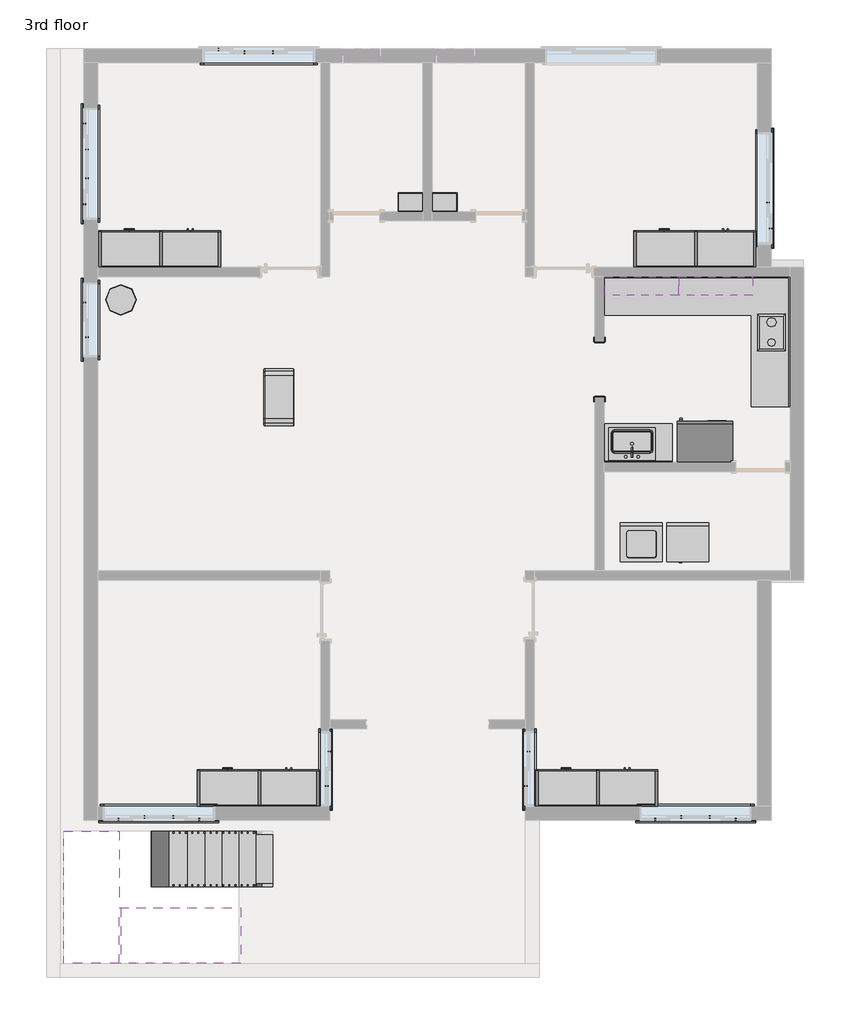
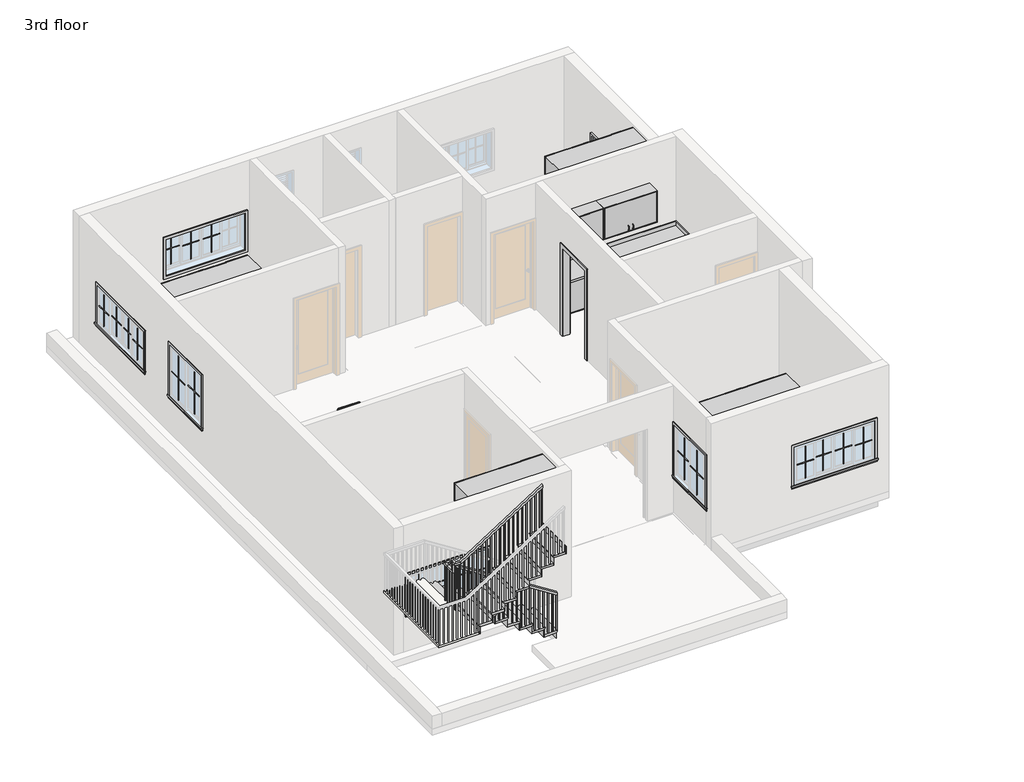
# One storey, part 3 of 4: 42 proxies, 15 furniture elements, 3 flow terminals, 2 stair flights, 1 railing, 1 slab.
"""IFC4 building model written with IfcOpenShell, lengths in millimetres."""

from ifc_helpers import new_model, si_unit, frame, origin, place, context, project, spatial, polyline, outline, extrude, faceted_brep, transform, mapped, element, save
from components import proxy_3c1fa1d0, proxy_97c73763, muntin_pattern_2x2_muntin_pattern_2x2_c2d27229, muntin_pattern_2x2_muntin_pattern_2x2_cf37b409, muntin_pattern_2x2_muntin_pattern_2x2_31a16349, proxy_7dd6dadb, trim_window_exterior_flat_with_sill_ac84ebb5, trim_window_exterior_flat_with_sill_7cfdd449, trim_window_exterior_flat_with_sill_3c945769, trim_window_interior_flat_picture_frame_caf2db4f, trim_window_interior_flat_picture_frame_f1e0b15b, trim_window_interior_flat_picture_frame_0edfbaa2, proxy_e75280ca, flow_terminal_7145266d, flow_terminal_4d548711, furniture_2dca108f, furniture_65fa61b5, furniture_1wardrobe_6271_1wardrobe_6271_4dd35231, furniture_3428e43d, furniture_bf8a676d, furniture_97fe820d, furniture_a6d59748, furniture_f5a42f9b, furniture_9d41381f, furniture_ea954fa4, non_monolithic_landing_543f77e1, stair_flight_6f06193a, stair_flight_13cb1edf

model = new_model("IFC4")

# Units and contexts
model_context = context("Model", 3, world=origin())
ifc_project = project(units=[si_unit("LENGTHUNIT", "METRE", prefix="MILLI")], contexts=[model_context])

# Site, building, storey
site = spatial("IfcSite", under=ifc_project)
building = spatial("IfcBuilding", under=site)
storey = spatial("IfcBuildingStorey", under=building, Name="3rd floor", Elevation=10210.8)

# Proxies
placement = place(None, origin())
proxy_shape = proxy_3c1fa1d0(model_context)
element("IfcBuildingElementProxy", 1, Name="Cook Top-2 Unit : 12\" x 18\" 2", ObjectType="Cook Top-2 Unit : 12\" x 18\" 2", at=placement, inside=storey, context=model_context, shape_type="MappedRepresentation", body=[
    mapped(proxy_shape, transform((-1440.8124084, 5502.3713848, 10210.8), x_axis=(1.0, 0.0, 0.0), y_axis=(0.0, 1.0, 0.0), z_axis=(0.0, 0.0, 1.0))),
])
proxy_2_shape = proxy_97c73763(model_context)
element("IfcBuildingElementProxy", 2, Name="Dryer : 27\" x 25\" x 35\"", ObjectType="Dryer : 27\" x 25\" x 35\"", at=placement, inside=storey, context=model_context, shape_type="MappedRepresentation", body=[
    mapped(proxy_2_shape, transform((-3115.1998647, 1776.2351766, 10210.8), x_axis=(1.0, 0.0, 0.0), y_axis=(0.0, 1.0, 0.0), z_axis=(0.0, 0.0, 1.0))),
])
muntin_pattern_2x2_muntin_pattern_2x2_shape = muntin_pattern_2x2_muntin_pattern_2x2_c2d27229(model_context)
element("IfcBuildingElementProxy", 3, Name="Muntin Pattern_2x2 : Muntin Pattern_2x2", ObjectType="Muntin Pattern_2x2 : Muntin Pattern_2x2", at=placement, inside=storey, context=model_context, shape_type="MappedRepresentation", body=[
    mapped(muntin_pattern_2x2_muntin_pattern_2x2_shape, transform((-12588.2374084, 5451.6336804, 11207.75), x_axis=(0.0, -1.0, 0.0), y_axis=(1.0, 0.0, 0.0), z_axis=(0.0, 0.0, 1.0))),
])
element("IfcBuildingElementProxy", 4, Name="Muntin Pattern_2x2 : Muntin Pattern_2x2", ObjectType="Muntin Pattern_2x2 : Muntin Pattern_2x2", at=placement, inside=storey, context=model_context, shape_type="MappedRepresentation", body=[
    mapped(muntin_pattern_2x2_muntin_pattern_2x2_shape, transform((-12632.6874084, 6019.9586804, 11207.75), x_axis=(0.0, -1.0, 0.0), y_axis=(1.0, 0.0, 0.0), z_axis=(0.0, 0.0, 1.0))),
])
muntin_pattern_2x2_muntin_pattern_2x2_2_shape = muntin_pattern_2x2_muntin_pattern_2x2_cf37b409(model_context)
element("IfcBuildingElementProxy", 5, Name="Muntin Pattern_2x2 : Muntin Pattern_2x2", ObjectType="Muntin Pattern_2x2 : Muntin Pattern_2x2", at=placement, inside=storey, context=model_context, shape_type="MappedRepresentation", body=[
    mapped(muntin_pattern_2x2_muntin_pattern_2x2_2_shape, transform((-8657.5874084, -1908.0163196, 11207.75), x_axis=(0.0, -1.0, 0.0), y_axis=(1.0, 0.0, 0.0), z_axis=(0.0, 0.0, 1.0))),
])
element("IfcBuildingElementProxy", 6, Name="Muntin Pattern_2x2 : Muntin Pattern_2x2", ObjectType="Muntin Pattern_2x2 : Muntin Pattern_2x2", at=placement, inside=storey, context=model_context, shape_type="MappedRepresentation", body=[
    mapped(muntin_pattern_2x2_muntin_pattern_2x2_2_shape, transform((-8613.1374084, -1339.6913196, 11207.75), x_axis=(0.0, -1.0, 0.0), y_axis=(1.0, 0.0, 0.0), z_axis=(0.0, 0.0, 1.0))),
])
element("IfcBuildingElementProxy", 7, Name="Muntin Pattern_2x2 : Muntin Pattern_2x2", ObjectType="Muntin Pattern_2x2 : Muntin Pattern_2x2", at=placement, inside=storey, context=model_context, shape_type="MappedRepresentation", body=[
    mapped(muntin_pattern_2x2_muntin_pattern_2x2_2_shape, transform((-5349.2374084, -1339.6913196, 11207.75), x_axis=(0.0, 1.0, 0.0), y_axis=(-1.0, 0.0, 0.0), z_axis=(0.0, 0.0, 1.0))),
])
element("IfcBuildingElementProxy", 8, Name="Muntin Pattern_2x2 : Muntin Pattern_2x2", ObjectType="Muntin Pattern_2x2 : Muntin Pattern_2x2", at=placement, inside=storey, context=model_context, shape_type="MappedRepresentation", body=[
    mapped(muntin_pattern_2x2_muntin_pattern_2x2_2_shape, transform((-5393.6874084, -1908.0163196, 11207.75), x_axis=(0.0, 1.0, 0.0), y_axis=(-1.0, 0.0, 0.0), z_axis=(0.0, 0.0, 1.0))),
])
muntin_pattern_2x2_muntin_pattern_2x2_3_shape = muntin_pattern_2x2_muntin_pattern_2x2_31a16349(model_context)
element("IfcBuildingElementProxy", 9, Name="Muntin Pattern_2x2 : Muntin Pattern_2x2", ObjectType="Muntin Pattern_2x2 : Muntin Pattern_2x2", at=placement, inside=storey, context=model_context, shape_type="MappedRepresentation", body=[
    mapped(muntin_pattern_2x2_muntin_pattern_2x2_3_shape, transform((-10432.4124084, 10171.2711804, 11207.75), x_axis=(1.0, 0.0, 0.0), y_axis=(0.0, 1.0, 0.0), z_axis=(0.0, 0.0, 1.0))),
])
element("IfcBuildingElementProxy", 10, Name="Muntin Pattern_2x2 : Muntin Pattern_2x2", ObjectType="Muntin Pattern_2x2 : Muntin Pattern_2x2", at=placement, inside=storey, context=model_context, shape_type="MappedRepresentation", body=[
    mapped(muntin_pattern_2x2_muntin_pattern_2x2_3_shape, transform((-10006.9624084, 10126.8211804, 11207.75), x_axis=(1.0, 0.0, 0.0), y_axis=(0.0, 1.0, 0.0), z_axis=(0.0, 0.0, 1.0))),
])
element("IfcBuildingElementProxy", 11, Name="Muntin Pattern_2x2 : Muntin Pattern_2x2", ObjectType="Muntin Pattern_2x2 : Muntin Pattern_2x2", at=placement, inside=storey, context=model_context, shape_type="MappedRepresentation", body=[
    mapped(muntin_pattern_2x2_muntin_pattern_2x2_3_shape, transform((-9537.0624084, 10126.8211804, 11207.75), x_axis=(1.0, 0.0, 0.0), y_axis=(0.0, 1.0, 0.0), z_axis=(0.0, 0.0, 1.0))),
])
element("IfcBuildingElementProxy", 12, Name="Muntin Pattern_2x2 : Muntin Pattern_2x2", ObjectType="Muntin Pattern_2x2 : Muntin Pattern_2x2", at=placement, inside=storey, context=model_context, shape_type="MappedRepresentation", body=[
    mapped(muntin_pattern_2x2_muntin_pattern_2x2_3_shape, transform((-12632.6874084, 7634.4461804, 11207.75), x_axis=(0.0, 1.0, 0.0), y_axis=(-1.0, 0.0, 0.0), z_axis=(0.0, 0.0, 1.0))),
])
element("IfcBuildingElementProxy", 13, Name="Muntin Pattern_2x2 : Muntin Pattern_2x2", ObjectType="Muntin Pattern_2x2 : Muntin Pattern_2x2", at=placement, inside=storey, context=model_context, shape_type="MappedRepresentation", body=[
    mapped(muntin_pattern_2x2_muntin_pattern_2x2_3_shape, transform((-12588.2374084, 8059.8961804, 11207.75), x_axis=(0.0, 1.0, 0.0), y_axis=(-1.0, 0.0, 0.0), z_axis=(0.0, 0.0, 1.0))),
])
element("IfcBuildingElementProxy", 14, Name="Muntin Pattern_2x2 : Muntin Pattern_2x2", ObjectType="Muntin Pattern_2x2 : Muntin Pattern_2x2", at=placement, inside=storey, context=model_context, shape_type="MappedRepresentation", body=[
    mapped(muntin_pattern_2x2_muntin_pattern_2x2_3_shape, transform((-12588.2374084, 8529.7961804, 11207.75), x_axis=(0.0, 1.0, 0.0), y_axis=(-1.0, 0.0, 0.0), z_axis=(0.0, 0.0, 1.0))),
])
element("IfcBuildingElementProxy", 15, Name="Muntin Pattern_2x2 : Muntin Pattern_2x2", ObjectType="Muntin Pattern_2x2 : Muntin Pattern_2x2", at=placement, inside=storey, context=model_context, shape_type="MappedRepresentation", body=[
    mapped(muntin_pattern_2x2_muntin_pattern_2x2_3_shape, transform((-12632.6874084, 8955.2461804, 11207.75), x_axis=(0.0, 1.0, 0.0), y_axis=(-1.0, 0.0, 0.0), z_axis=(0.0, 0.0, 1.0))),
])
element("IfcBuildingElementProxy", 16, Name="Muntin Pattern_2x2 : Muntin Pattern_2x2", ObjectType="Muntin Pattern_2x2 : Muntin Pattern_2x2", at=placement, inside=storey, context=model_context, shape_type="MappedRepresentation", body=[
    mapped(muntin_pattern_2x2_muntin_pattern_2x2_3_shape, transform((-1418.5874084, 7659.8461804, 11207.75), x_axis=(0.0, -1.0, 0.0), y_axis=(1.0, 0.0, 0.0), z_axis=(0.0, 0.0, 1.0))),
])
element("IfcBuildingElementProxy", 17, Name="Muntin Pattern_2x2 : Muntin Pattern_2x2", ObjectType="Muntin Pattern_2x2 : Muntin Pattern_2x2", at=placement, inside=storey, context=model_context, shape_type="MappedRepresentation", body=[
    mapped(muntin_pattern_2x2_muntin_pattern_2x2_3_shape, transform((-1374.1374084, 7234.3961804, 11207.75), x_axis=(0.0, -1.0, 0.0), y_axis=(1.0, 0.0, 0.0), z_axis=(0.0, 0.0, 1.0))),
])
element("IfcBuildingElementProxy", 18, Name="Muntin Pattern_2x2 : Muntin Pattern_2x2", ObjectType="Muntin Pattern_2x2 : Muntin Pattern_2x2", at=placement, inside=storey, context=model_context, shape_type="MappedRepresentation", body=[
    mapped(muntin_pattern_2x2_muntin_pattern_2x2_3_shape, transform((-1948.8124084, -2458.8788196, 11207.75), x_axis=(-1.0, 0.0, 0.0), y_axis=(0.0, -1.0, 0.0), z_axis=(0.0, 0.0, 1.0))),
])
element("IfcBuildingElementProxy", 19, Name="Muntin Pattern_2x2 : Muntin Pattern_2x2", ObjectType="Muntin Pattern_2x2 : Muntin Pattern_2x2", at=placement, inside=storey, context=model_context, shape_type="MappedRepresentation", body=[
    mapped(muntin_pattern_2x2_muntin_pattern_2x2_3_shape, transform((-2374.2624084, -2414.4288196, 11207.75), x_axis=(-1.0, 0.0, 0.0), y_axis=(0.0, -1.0, 0.0), z_axis=(0.0, 0.0, 1.0))),
])
element("IfcBuildingElementProxy", 20, Name="Muntin Pattern_2x2 : Muntin Pattern_2x2", ObjectType="Muntin Pattern_2x2 : Muntin Pattern_2x2", at=placement, inside=storey, context=model_context, shape_type="MappedRepresentation", body=[
    mapped(muntin_pattern_2x2_muntin_pattern_2x2_3_shape, transform((-2844.1624084, -2414.4288196, 11207.75), x_axis=(-1.0, 0.0, 0.0), y_axis=(0.0, -1.0, 0.0), z_axis=(0.0, 0.0, 1.0))),
])
element("IfcBuildingElementProxy", 21, Name="Muntin Pattern_2x2 : Muntin Pattern_2x2", ObjectType="Muntin Pattern_2x2 : Muntin Pattern_2x2", at=placement, inside=storey, context=model_context, shape_type="MappedRepresentation", body=[
    mapped(muntin_pattern_2x2_muntin_pattern_2x2_3_shape, transform((-3269.6124084, -2458.8788196, 11207.75), x_axis=(-1.0, 0.0, 0.0), y_axis=(0.0, -1.0, 0.0), z_axis=(0.0, 0.0, 1.0))),
])
element("IfcBuildingElementProxy", 22, Name="Muntin Pattern_2x2 : Muntin Pattern_2x2", ObjectType="Muntin Pattern_2x2 : Muntin Pattern_2x2", at=placement, inside=storey, context=model_context, shape_type="MappedRepresentation", body=[
    mapped(muntin_pattern_2x2_muntin_pattern_2x2_3_shape, transform((-10749.9124084, -2458.8788196, 11207.75), x_axis=(-1.0, 0.0, 0.0), y_axis=(0.0, -1.0, 0.0), z_axis=(0.0, 0.0, 1.0))),
])
element("IfcBuildingElementProxy", 23, Name="Muntin Pattern_2x2 : Muntin Pattern_2x2", ObjectType="Muntin Pattern_2x2 : Muntin Pattern_2x2", at=placement, inside=storey, context=model_context, shape_type="MappedRepresentation", body=[
    mapped(muntin_pattern_2x2_muntin_pattern_2x2_3_shape, transform((-11175.3624084, -2414.4288196, 11207.75), x_axis=(-1.0, 0.0, 0.0), y_axis=(0.0, -1.0, 0.0), z_axis=(0.0, 0.0, 1.0))),
])
element("IfcBuildingElementProxy", 24, Name="Muntin Pattern_2x2 : Muntin Pattern_2x2", ObjectType="Muntin Pattern_2x2 : Muntin Pattern_2x2", at=placement, inside=storey, context=model_context, shape_type="MappedRepresentation", body=[
    mapped(muntin_pattern_2x2_muntin_pattern_2x2_3_shape, transform((-11645.2624084, -2414.4288196, 11207.75), x_axis=(-1.0, 0.0, 0.0), y_axis=(0.0, -1.0, 0.0), z_axis=(0.0, 0.0, 1.0))),
])
element("IfcBuildingElementProxy", 25, Name="Muntin Pattern_2x2 : Muntin Pattern_2x2", ObjectType="Muntin Pattern_2x2 : Muntin Pattern_2x2", at=placement, inside=storey, context=model_context, shape_type="MappedRepresentation", body=[
    mapped(muntin_pattern_2x2_muntin_pattern_2x2_3_shape, transform((-12070.7124084, -2458.8788196, 11207.75), x_axis=(-1.0, 0.0, 0.0), y_axis=(0.0, -1.0, 0.0), z_axis=(0.0, 0.0, 1.0))),
])
proxy_3_shape = proxy_7dd6dadb(model_context)
element("IfcBuildingElementProxy", 26, Name="Passage Opening-Cased : 36\" x 84\"", ObjectType="Passage Opening-Cased : 36\" x 84\"", at=placement, inside=storey, context=model_context, shape_type="MappedRepresentation", body=[
    mapped(proxy_3_shape, transform((-4184.0124084, 4931.1848371, 10210.8), x_axis=(0.0, 1.0, 0.0), y_axis=(-1.0, 0.0, 0.0), z_axis=(0.0, 0.0, 1.0))),
])
trim_window_exterior_flat_with_sill_shape = trim_window_exterior_flat_with_sill_ac84ebb5(model_context)
element("IfcBuildingElementProxy", 27, Name="Trim-Window-Exterior-Flat : with Sill", ObjectType="Trim-Window-Exterior-Flat : with Sill", at=placement, inside=storey, context=model_context, shape_type="MappedRepresentation", body=[
    mapped(trim_window_exterior_flat_with_sill_shape, transform((-12642.2124084, 5735.7961804, 12344.4), x_axis=(0.0, 1.0, 0.0), y_axis=(0.0, 0.0, -1.0), z_axis=(-1.0, 0.0, 0.0))),
])
trim_window_exterior_flat_with_sill_2_shape = trim_window_exterior_flat_with_sill_7cfdd449(model_context)
element("IfcBuildingElementProxy", 28, Name="Trim-Window-Exterior-Flat : with Sill", ObjectType="Trim-Window-Exterior-Flat : with Sill", at=placement, inside=storey, context=model_context, shape_type="MappedRepresentation", body=[
    mapped(trim_window_exterior_flat_with_sill_2_shape, transform((-8603.6124084, -1623.8538196, 12344.4), x_axis=(0.0, 1.0, 0.0), y_axis=(0.0, 0.0, 1.0), z_axis=(1.0, 0.0, 0.0))),
])
element("IfcBuildingElementProxy", 29, Name="Trim-Window-Exterior-Flat : with Sill", ObjectType="Trim-Window-Exterior-Flat : with Sill", at=placement, inside=storey, context=model_context, shape_type="MappedRepresentation", body=[
    mapped(trim_window_exterior_flat_with_sill_2_shape, transform((-5403.2124084, -1623.8538196, 12344.4), x_axis=(0.0, -1.0, 0.0), y_axis=(0.0, 0.0, 1.0), z_axis=(-1.0, 0.0, 0.0))),
])
trim_window_exterior_flat_with_sill_3_shape = trim_window_exterior_flat_with_sill_3c945769(model_context)
element("IfcBuildingElementProxy", 30, Name="Trim-Window-Exterior-Flat : with Sill", ObjectType="Trim-Window-Exterior-Flat : with Sill", at=placement, inside=storey, context=model_context, shape_type="MappedRepresentation", body=[
    mapped(trim_window_exterior_flat_with_sill_3_shape, transform((-12642.2124084, 8294.8461804, 12039.6), x_axis=(0.0, -1.0, 0.0), y_axis=(0.0, 0.0, 1.0), z_axis=(-1.0, 0.0, 0.0))),
])
element("IfcBuildingElementProxy", 31, Name="Trim-Window-Exterior-Flat : with Sill", ObjectType="Trim-Window-Exterior-Flat : with Sill", at=placement, inside=storey, context=model_context, shape_type="MappedRepresentation", body=[
    mapped(trim_window_exterior_flat_with_sill_3_shape, transform((-1364.6124084, 7894.7961804, 12039.6), x_axis=(0.0, 1.0, 0.0), y_axis=(0.0, 0.0, 1.0), z_axis=(1.0, 0.0, 0.0))),
])
element("IfcBuildingElementProxy", 32, Name="Trim-Window-Exterior-Flat : with Sill", ObjectType="Trim-Window-Exterior-Flat : with Sill", at=placement, inside=storey, context=model_context, shape_type="MappedRepresentation", body=[
    mapped(trim_window_exterior_flat_with_sill_3_shape, transform((-2609.2124084, -2468.4038196, 12039.6), x_axis=(1.0, 0.0, 0.0), y_axis=(0.0, 0.0, 1.0), z_axis=(0.0, -1.0, 0.0))),
])
element("IfcBuildingElementProxy", 33, Name="Trim-Window-Exterior-Flat : with Sill", ObjectType="Trim-Window-Exterior-Flat : with Sill", at=placement, inside=storey, context=model_context, shape_type="MappedRepresentation", body=[
    mapped(trim_window_exterior_flat_with_sill_3_shape, transform((-11410.3124084, -2468.4038196, 12039.6), x_axis=(1.0, 0.0, 0.0), y_axis=(0.0, 0.0, 1.0), z_axis=(0.0, -1.0, 0.0))),
])
trim_window_interior_flat_picture_frame_shape = trim_window_interior_flat_picture_frame_caf2db4f(model_context)
element("IfcBuildingElementProxy", 34, Name="Trim-Window-Interior-Flat : Picture Frame", ObjectType="Trim-Window-Interior-Flat : Picture Frame", at=placement, inside=storey, context=model_context, shape_type="MappedRepresentation", body=[
    mapped(trim_window_interior_flat_picture_frame_shape, transform((-12413.6124084, 5735.7961804, 12344.4), x_axis=(0.0, -1.0, 0.0), y_axis=(0.0, 0.0, -1.0), z_axis=(1.0, 0.0, 0.0))),
])
trim_window_interior_flat_picture_frame_2_shape = trim_window_interior_flat_picture_frame_f1e0b15b(model_context)
element("IfcBuildingElementProxy", 35, Name="Trim-Window-Interior-Flat : Picture Frame", ObjectType="Trim-Window-Interior-Flat : Picture Frame", at=placement, inside=storey, context=model_context, shape_type="MappedRepresentation", body=[
    mapped(trim_window_interior_flat_picture_frame_2_shape, transform((-8756.0124084, -1623.8538196, 12344.4), x_axis=(0.0, -1.0, 0.0), y_axis=(0.0, 0.0, 1.0), z_axis=(-1.0, 0.0, 0.0))),
])
element("IfcBuildingElementProxy", 36, Name="Trim-Window-Interior-Flat : Picture Frame", ObjectType="Trim-Window-Interior-Flat : Picture Frame", at=placement, inside=storey, context=model_context, shape_type="MappedRepresentation", body=[
    mapped(trim_window_interior_flat_picture_frame_2_shape, transform((-5250.8124084, -1623.8538196, 12344.4), x_axis=(0.0, 1.0, 0.0), y_axis=(0.0, 0.0, 1.0), z_axis=(1.0, 0.0, 0.0))),
])
trim_window_interior_flat_picture_frame_3_shape = trim_window_interior_flat_picture_frame_0edfbaa2(model_context)
element("IfcBuildingElementProxy", 37, Name="Trim-Window-Interior-Flat : Picture Frame", ObjectType="Trim-Window-Interior-Flat : Picture Frame", at=placement, inside=storey, context=model_context, shape_type="MappedRepresentation", body=[
    mapped(trim_window_interior_flat_picture_frame_3_shape, transform((-9772.0124084, 9952.1961804, 12039.6), x_axis=(1.0, 0.0, 0.0), y_axis=(0.0, 0.0, 1.0), z_axis=(0.0, -1.0, 0.0))),
])
element("IfcBuildingElementProxy", 38, Name="Trim-Window-Interior-Flat : Picture Frame", ObjectType="Trim-Window-Interior-Flat : Picture Frame", at=placement, inside=storey, context=model_context, shape_type="MappedRepresentation", body=[
    mapped(trim_window_interior_flat_picture_frame_3_shape, transform((-12413.6124084, 8294.8461804, 12039.6), x_axis=(0.0, 1.0, 0.0), y_axis=(0.0, 0.0, 1.0), z_axis=(1.0, 0.0, 0.0))),
])
element("IfcBuildingElementProxy", 39, Name="Trim-Window-Interior-Flat : Picture Frame", ObjectType="Trim-Window-Interior-Flat : Picture Frame", at=placement, inside=storey, context=model_context, shape_type="MappedRepresentation", body=[
    mapped(trim_window_interior_flat_picture_frame_3_shape, transform((-1593.2124084, 7894.7961804, 12039.6), x_axis=(0.0, -1.0, 0.0), y_axis=(0.0, 0.0, 1.0), z_axis=(-1.0, 0.0, 0.0))),
])
element("IfcBuildingElementProxy", 40, Name="Trim-Window-Interior-Flat : Picture Frame", ObjectType="Trim-Window-Interior-Flat : Picture Frame", at=placement, inside=storey, context=model_context, shape_type="MappedRepresentation", body=[
    mapped(trim_window_interior_flat_picture_frame_3_shape, transform((-2609.2124084, -2239.8038196, 12039.6), x_axis=(-1.0, 0.0, 0.0), y_axis=(0.0, 0.0, 1.0), z_axis=(0.0, 1.0, 0.0))),
])
element("IfcBuildingElementProxy", 41, Name="Trim-Window-Interior-Flat : Picture Frame", ObjectType="Trim-Window-Interior-Flat : Picture Frame", at=placement, inside=storey, context=model_context, shape_type="MappedRepresentation", body=[
    mapped(trim_window_interior_flat_picture_frame_3_shape, transform((-11410.3124084, -2239.8038196, 12039.6), x_axis=(-1.0, 0.0, 0.0), y_axis=(0.0, 0.0, 1.0), z_axis=(0.0, 1.0, 0.0))),
])
proxy_4_shape = proxy_e75280ca(model_context)
element("IfcBuildingElementProxy", 42, Name="Washer : 27\" x 25\" x 35\"", ObjectType="Washer : 27\" x 25\" x 35\"", at=placement, inside=storey, context=model_context, shape_type="MappedRepresentation", body=[
    mapped(proxy_4_shape, transform((-3918.6298768, 1811.7466156, 10210.8), x_axis=(1.0, 0.0, 0.0), y_axis=(0.0, 1.0, 0.0), z_axis=(0.0, 0.0, 1.0))),
])

# Flow terminals
flow_terminal_shape = flow_terminal_7145266d(model_context)
element("IfcFlowTerminal", 43, ObjectType="Sink - Work : 20\"x18\" 2", at=placement, inside=storey, context=model_context, shape_type="MappedRepresentation", body=[
    mapped(flow_terminal_shape, transform((-7282.8124084, 7513.7961804, 11125.2), x_axis=(-1.0, 0.0, 0.0), y_axis=(0.0, -1.0, 0.0), z_axis=(0.0, 0.0, 1.0))),
])
element("IfcFlowTerminal", 44, ObjectType="Sink - Work : 20\"x18\" 2", at=placement, inside=storey, context=model_context, shape_type="MappedRepresentation", body=[
    mapped(flow_terminal_shape, transform((-6724.0124084, 7513.7961804, 11125.2), x_axis=(-1.0, 0.0, 0.0), y_axis=(0.0, -1.0, 0.0), z_axis=(0.0, 0.0, 1.0))),
])
flow_terminal_2_shape = flow_terminal_4d548711(model_context)
element("IfcFlowTerminal", 45, ObjectType="Sink Kitchen-Single : 30\" x 21\"", at=placement, inside=storey, context=model_context, shape_type="MappedRepresentation", body=[
    mapped(flow_terminal_2_shape, transform((-3634.9231678, 3706.1415815, 10210.8), x_axis=(-1.0, 0.0, 0.0), y_axis=(0.0, -1.0, 0.0), z_axis=(0.0, 0.0, 1.0))),
])

# Furniture
furniture_shape = furniture_2dca108f(model_context)
element("IfcFurniture", 46, at=placement, inside=storey, context=model_context, shape_type="MappedRepresentation", body=[
    mapped(furniture_shape, transform((-9441.8124084, 4465.7961804, 10210.8), x_axis=(1.0, 0.0, 0.0), y_axis=(0.0, 1.0, 0.0), z_axis=(0.0, 0.0, 1.0))),
])
furniture_2_shape = furniture_65fa61b5(model_context)
element("IfcFurniture", 47, at=placement, inside=storey, context=model_context, shape_type="MappedRepresentation", body=[
    mapped(furniture_2_shape, transform((-3066.4124084, 3411.6961804, 10210.8), x_axis=(-1.0, 0.0, 0.0), y_axis=(0.0, -1.0, 0.0), z_axis=(0.0, 0.0, 1.0))),
])
furniture_1wardrobe_6271_1wardrobe_6271_shape = furniture_1wardrobe_6271_1wardrobe_6271_4dd35231(model_context)
element("IfcFurniture", 48, ObjectType="1Wardrobe_6271 : 1Wardrobe_6271", at=placement, inside=storey, context=model_context, shape_type="MappedRepresentation", body=[
    mapped(furniture_1wardrobe_6271_1wardrobe_6271_shape, transform((-10394.3124084, 6599.3961804, 10210.8), x_axis=(-1.0, 0.0, 0.0), y_axis=(0.0, -1.0, 0.0), z_axis=(0.0, 0.0, 1.0))),
])
element("IfcFurniture", 49, ObjectType="1Wardrobe_6271 : 1Wardrobe_6271", at=placement, inside=storey, context=model_context, shape_type="MappedRepresentation", body=[
    mapped(furniture_1wardrobe_6271_1wardrobe_6271_shape, transform((-1618.6124084, 6599.3961804, 10210.8), x_axis=(-1.0, 0.0, 0.0), y_axis=(0.0, -1.0, 0.0), z_axis=(0.0, 0.0, 1.0))),
])
element("IfcFurniture", 50, ObjectType="1Wardrobe_6271 : 1Wardrobe_6271", at=placement, inside=storey, context=model_context, shape_type="MappedRepresentation", body=[
    mapped(furniture_1wardrobe_6271_1wardrobe_6271_shape, transform((-3231.5124084, -2239.8038196, 10210.8), x_axis=(-1.0, 0.0, 0.0), y_axis=(0.0, -1.0, 0.0), z_axis=(0.0, 0.0, 1.0))),
])
element("IfcFurniture", 51, ObjectType="1Wardrobe_6271 : 1Wardrobe_6271", at=placement, inside=storey, context=model_context, shape_type="MappedRepresentation", body=[
    mapped(furniture_1wardrobe_6271_1wardrobe_6271_shape, transform((-8781.4124084, -2239.8038196, 10210.8), x_axis=(-1.0, 0.0, 0.0), y_axis=(0.0, -1.0, 0.0), z_axis=(0.0, 0.0, 1.0))),
])
furniture_3_shape = furniture_3428e43d(model_context)
element("IfcFurniture", 52, ObjectType="48\" 2", at=placement, inside=storey, context=model_context, shape_type="MappedRepresentation", body=[
    mapped(furniture_3_shape, transform((-2674.6573683, 6446.9961804, 10210.8), x_axis=(1.0, 0.0, 0.0), y_axis=(0.0, 1.0, 0.0), z_axis=(0.0, 0.0, 1.0))),
])
element("IfcFurniture", 53, ObjectType="48\" 3", at=placement, inside=storey, context=model_context, shape_type="MappedRepresentation", body=[
    mapped(furniture_3_shape, transform((-1059.8124084, 5013.8411403, 10210.8), x_axis=(0.0, -1.0, 0.0), y_axis=(1.0, 0.0, 0.0), z_axis=(0.0, 0.0, 1.0))),
])
furniture_4_shape = furniture_bf8a676d(model_context)
element("IfcFurniture", 54, ObjectType="Base Cabinet-Combo01 : 30\" 2", at=placement, inside=storey, context=model_context, shape_type="MappedRepresentation", body=[
    mapped(furniture_4_shape, transform((-3669.3501133, 6446.9961804, 10210.8), x_axis=(1.0, 0.0, 0.0), y_axis=(0.0, 1.0, 0.0), z_axis=(0.0, 0.0, 1.0))),
])
furniture_5_shape = furniture_97fe820d(model_context)
element("IfcFurniture", 55, ObjectType="Base Cabinet-Corner Unit-Square : 36\"", at=placement, inside=storey, context=model_context, shape_type="MappedRepresentation", body=[
    mapped(furniture_5_shape, transform((-1586.5501133, 6446.9961804, 10210.8), x_axis=(1.0, 0.0, 0.0), y_axis=(0.0, 1.0, 0.0), z_axis=(0.0, 0.0, 1.0))),
])
furniture_6_shape = furniture_a6d59748(model_context)
element("IfcFurniture", 56, ObjectType="Counter Top w Sink Hole : 24\" Depth", at=placement, inside=storey, context=model_context, shape_type="MappedRepresentation", body=[
    mapped(furniture_6_shape, transform((-4190.6747034, 3398.9961804, 10210.8), x_axis=(-1.0, 0.0, 0.0), y_axis=(0.0, -1.0, 0.0), z_axis=(0.0, 0.0, 1.0))),
])
furniture_7_shape = furniture_f5a42f9b(model_context)
element("IfcFurniture", 57, ObjectType="Counter Top-L Shaped : 24\" Depth", at=placement, inside=storey, context=model_context, shape_type="MappedRepresentation", body=[
    mapped(furniture_7_shape, transform((-1059.8124084, 5246.5338853, 10210.8), x_axis=(0.0, -1.0, 0.0), y_axis=(1.0, 0.0, 0.0), z_axis=(0.0, 0.0, 1.0))),
])
furniture_8_shape = furniture_9d41381f(model_context)
element("IfcFurniture", 58, ObjectType="Table-Trio End : 20\" Diameter", at=placement, inside=storey, context=model_context, shape_type="MappedRepresentation", body=[
    mapped(furniture_8_shape, transform((-12032.6124084, 6065.9961804, 10210.8), x_axis=(1.0, 0.0, 0.0), y_axis=(0.0, 1.0, 0.0), z_axis=(0.0, 0.0, 1.0))),
])
furniture_9_shape = furniture_ea954fa4(model_context)
element("IfcFurniture", 59, ObjectType="Upper Cabinet-Pass-Thru : 48\" x 30\" x 12\"", at=placement, inside=storey, context=model_context, shape_type="MappedRepresentation", body=[
    mapped(furniture_9_shape, transform((-3516.9501133, 6446.9961804, 10210.8), x_axis=(1.0, 0.0, 0.0), y_axis=(0.0, 1.0, 0.0), z_axis=(0.0, 0.0, 1.0))),
])
element("IfcFurniture", 60, ObjectType="Upper Cabinet-Pass-Thru : 48\" x 30\" x 12\"", at=placement, inside=storey, context=model_context, shape_type="MappedRepresentation", body=[
    mapped(furniture_9_shape, transform((-2297.7501133, 6446.9961804, 10210.8), x_axis=(1.0, 0.0, 0.0), y_axis=(0.0, 1.0, 0.0), z_axis=(0.0, 0.0, 1.0))),
])

# Railing
element("IfcRailing", 61, ObjectType="Handrail - Rectangular", at=placement, inside=storey, context=model_context, shape_type="SolidModel", body=[
    faceted_brep([(-9543.8120641, -3562.3669819, 11303.0), (-9543.8120641, -3562.3669819, 11242.786276), (-9543.8120641, -3511.5669819, 11242.786276), (-9543.8120641, -3511.5669819, 11303.0), (-11982.2120641, -3562.3669819, 12854.7090909), (-12033.0120641, -3562.3669819, 12826.8226396), (-12033.0120641, -3511.5669819, 12826.8226396), (-11982.2120641, -3511.5669819, 12854.7090909), (-11982.2120641, -3562.3669819, 12903.2), (-12033.0120641, -3562.3669819, 12852.4), (-12033.0120641, -3511.5669819, 12852.4), (-11982.2120641, -3511.5669819, 12903.2), (-12058.4120641, -3562.3669819, 12903.2), (-12058.4120641, -3562.3669819, 12852.4), (-12109.2120641, -3511.5669819, 12852.4), (-12109.2120641, -3511.5669819, 12903.2), (-12058.4120641, -3638.5669819, 12903.2), (-12058.4120641, -3638.5669819, 12852.4), (-12109.2120641, -3638.5669819, 12852.4), (-12109.2120641, -3638.5669819, 12903.2), (-12058.4120641, -3827.3038196, 12903.2), (-12058.4120641, -3878.1038196, 12852.4), (-12109.2120641, -3878.1038196, 12852.4), (-12109.2120641, -3827.3038196, 12903.2), (-12058.4120641, -3827.3038196, 13129.4909091), (-12058.4120641, -3878.1038196, 13078.6909091), (-12109.2120641, -3878.1038196, 13078.6909091), (-12109.2120641, -3827.3038196, 13129.4909091), (-12058.4120641, -3903.5038196, 13129.4909091), (-12058.4120641, -3903.5038196, 13078.6909091), (-12109.2120641, -3954.3038196, 13078.6909091), (-12109.2120641, -3954.3038196, 13129.4909091), (-11982.2120641, -3903.5038196, 13129.4909091), (-11967.4190691, -3903.5038196, 13078.6909091), (-11967.4190691, -3954.3038196, 13078.6909091), (-11982.2120641, -3954.3038196, 13129.4909091), (-10102.6120641, -3903.5038196, 14325.6), (-10102.6120641, -3954.3038196, 14325.6), (-10102.6120641, -3954.3038196, 14265.386276), (-10102.6120641, -3903.5038196, 14265.386276)], [[[0, 1, 2, 3]], [[1, 0, 4, 5]], [[2, 1, 5, 6]], [[3, 2, 6, 7]], [[0, 3, 7, 4]], [[5, 4, 8, 9]], [[6, 5, 9, 10]], [[7, 6, 10, 11]], [[4, 7, 11, 8]], [[9, 8, 12, 13]], [[10, 9, 13, 14]], [[11, 10, 14, 15]], [[8, 11, 15, 12]], [[13, 12, 16, 17]], [[14, 13, 17, 18]], [[15, 14, 18, 19]], [[12, 15, 19, 16]], [[17, 16, 20, 21]], [[18, 17, 21, 22]], [[19, 18, 22, 23]], [[16, 19, 23, 20]], [[21, 20, 24, 25]], [[22, 21, 25, 26]], [[23, 22, 26, 27]], [[20, 23, 27, 24]], [[25, 24, 28, 29]], [[26, 25, 29, 30]], [[27, 26, 30, 31]], [[24, 27, 31, 28]], [[29, 28, 32, 33]], [[30, 29, 33, 34]], [[31, 30, 34, 35]], [[28, 31, 35, 32]], [[36, 37, 38, 39]], [[33, 32, 36, 39]], [[34, 33, 39, 38]], [[35, 34, 38, 37]], [[32, 35, 37, 36]]]),
    extrude(outline(polyline([(14226.9976396, -10162.9370641), (13233.4, -10162.9370641), (13233.4, -10143.8870641), (14239.1203669, -10143.8870641), (14226.9976396, -10162.9370641)])), frame((0.0, -3938.4288196, 0.0), z_axis=(0.0, 1.0, 0.0), x_axis=(0.0, 0.0, 1.0)), (0.0, 0.0, 1.0), 19.05),
    extrude(outline(polyline([(14162.3430941, -10264.5370641), (13233.4, -10264.5370641), (13233.4, -10245.4870641), (14174.4658214, -10245.4870641), (14162.3430941, -10264.5370641)])), frame((0.0, -3938.4288196, 0.0), z_axis=(0.0, 1.0, 0.0), x_axis=(0.0, 0.0, 1.0)), (0.0, 0.0, 1.0), 19.05),
    extrude(outline(polyline([(14097.6885487, -10366.1370641), (13233.4, -10366.1370641), (13233.4, -10347.0870641), (14109.811276, -10347.0870641), (14097.6885487, -10366.1370641)])), frame((0.0, -3938.4288196, 0.0), z_axis=(0.0, 1.0, 0.0), x_axis=(0.0, 0.0, 1.0)), (0.0, 0.0, 1.0), 19.05),
    extrude(outline(polyline([(14033.0340032, -10467.7370641), (13055.6, -10467.7370641), (13055.6, -10448.6870641), (14045.1567305, -10448.6870641), (14033.0340032, -10467.7370641)])), frame((0.0, -3938.4288196, 0.0), z_axis=(0.0, 1.0, 0.0), x_axis=(0.0, 0.0, 1.0)), (0.0, 0.0, 1.0), 19.05),
    extrude(outline(polyline([(13968.3794578, -10569.3370641), (13055.6, -10569.3370641), (13055.6, -10550.2870641), (13980.5021851, -10550.2870641), (13968.3794578, -10569.3370641)])), frame((0.0, -3938.4288196, 0.0), z_axis=(0.0, 1.0, 0.0), x_axis=(0.0, 0.0, 1.0)), (0.0, 0.0, 1.0), 19.05),
    extrude(outline(polyline([(13903.7249123, -10670.9370641), (13055.6, -10670.9370641), (13055.6, -10651.8870641), (13915.8476396, -10651.8870641), (13903.7249123, -10670.9370641)])), frame((0.0, -3938.4288196, 0.0), z_axis=(0.0, 1.0, 0.0), x_axis=(0.0, 0.0, 1.0)), (0.0, 0.0, 1.0), 19.05),
    extrude(outline(polyline([(13839.0703669, -10772.5370641), (12877.8, -10772.5370641), (12877.8, -10753.4870641), (13851.1930941, -10753.4870641), (13839.0703669, -10772.5370641)])), frame((0.0, -3938.4288196, 0.0), z_axis=(0.0, 1.0, 0.0), x_axis=(0.0, 0.0, 1.0)), (0.0, 0.0, 1.0), 19.05),
    extrude(outline(polyline([(13774.4158214, -10874.1370641), (12877.8, -10874.1370641), (12877.8, -10855.0870641), (13786.5385487, -10855.0870641), (13774.4158214, -10874.1370641)])), frame((0.0, -3938.4288196, 0.0), z_axis=(0.0, 1.0, 0.0), x_axis=(0.0, 0.0, 1.0)), (0.0, 0.0, 1.0), 19.05),
    extrude(outline(polyline([(13709.761276, -10975.7370641), (12700.0, -10975.7370641), (12700.0, -10956.6870641), (13721.8840032, -10956.6870641), (13709.761276, -10975.7370641)])), frame((0.0, -3938.4288196, 0.0), z_axis=(0.0, 1.0, 0.0), x_axis=(0.0, 0.0, 1.0)), (0.0, 0.0, 1.0), 19.05),
    extrude(outline(polyline([(13645.1067305, -11077.3370641), (12700.0, -11077.3370641), (12700.0, -11058.2870641), (13657.2294578, -11058.2870641), (13645.1067305, -11077.3370641)])), frame((0.0, -3938.4288196, 0.0), z_axis=(0.0, 1.0, 0.0), x_axis=(0.0, 0.0, 1.0)), (0.0, 0.0, 1.0), 19.05),
    extrude(outline(polyline([(13580.4521851, -11178.9370641), (12700.0, -11178.9370641), (12700.0, -11159.8870641), (13592.5749123, -11159.8870641), (13580.4521851, -11178.9370641)])), frame((0.0, -3938.4288196, 0.0), z_axis=(0.0, 1.0, 0.0), x_axis=(0.0, 0.0, 1.0)), (0.0, 0.0, 1.0), 19.05),
    extrude(outline(polyline([(13515.7976396, -11280.5370641), (12522.2, -11280.5370641), (12522.2, -11261.4870641), (13527.9203669, -11261.4870641), (13515.7976396, -11280.5370641)])), frame((0.0, -3938.4288196, 0.0), z_axis=(0.0, 1.0, 0.0), x_axis=(0.0, 0.0, 1.0)), (0.0, 0.0, 1.0), 19.05),
    extrude(outline(polyline([(13451.1430941, -11382.1370641), (12522.2, -11382.1370641), (12522.2, -11363.0870641), (13463.2658214, -11363.0870641), (13451.1430941, -11382.1370641)])), frame((0.0, -3938.4288196, 0.0), z_axis=(0.0, 1.0, 0.0), x_axis=(0.0, 0.0, 1.0)), (0.0, 0.0, 1.0), 19.05),
    extrude(outline(polyline([(13386.4885487, -11483.7370641), (12522.2, -11483.7370641), (12522.2, -11464.6870641), (13398.611276, -11464.6870641), (13386.4885487, -11483.7370641)])), frame((0.0, -3938.4288196, 0.0), z_axis=(0.0, 1.0, 0.0), x_axis=(0.0, 0.0, 1.0)), (0.0, 0.0, 1.0), 19.05),
    extrude(outline(polyline([(13321.8340032, -11585.3370641), (12344.4, -11585.3370641), (12344.4, -11566.2870641), (13333.9567305, -11566.2870641), (13321.8340032, -11585.3370641)])), frame((0.0, -3938.4288196, 0.0), z_axis=(0.0, 1.0, 0.0), x_axis=(0.0, 0.0, 1.0)), (0.0, 0.0, 1.0), 19.05),
    extrude(outline(polyline([(13257.1794578, -11686.9370641), (12344.4, -11686.9370641), (12344.4, -11667.8870641), (13269.3021851, -11667.8870641), (13257.1794578, -11686.9370641)])), frame((0.0, -3938.4288196, 0.0), z_axis=(0.0, 1.0, 0.0), x_axis=(0.0, 0.0, 1.0)), (0.0, 0.0, 1.0), 19.05),
    extrude(outline(polyline([(13192.5249123, -11788.5370641), (12344.4, -11788.5370641), (12344.4, -11769.4870641), (13204.6476396, -11769.4870641), (13192.5249123, -11788.5370641)])), frame((0.0, -3938.4288196, 0.0), z_axis=(0.0, 1.0, 0.0), x_axis=(0.0, 0.0, 1.0)), (0.0, 0.0, 1.0), 19.05),
    extrude(outline(polyline([(13127.8703669, -11890.1370641), (12166.6, -11890.1370641), (12166.6, -11871.0870641), (13139.9930941, -11871.0870641), (13127.8703669, -11890.1370641)])), frame((0.0, -3938.4288196, 0.0), z_axis=(0.0, 1.0, 0.0), x_axis=(0.0, 0.0, 1.0)), (0.0, 0.0, 1.0), 19.05),
    extrude(outline(polyline([(13063.2158214, -11991.7370641), (12166.6, -11991.7370641), (12166.6, -11972.6870641), (13075.3385487, -11972.6870641), (13063.2158214, -11991.7370641)])), frame((0.0, -3938.4288196, 0.0), z_axis=(0.0, 1.0, 0.0), x_axis=(0.0, 0.0, 1.0)), (0.0, 0.0, 1.0), 19.05),
    extrude(outline(polyline([(-12074.2870641, -3832.2419819), (-12074.2870641, -3851.2919819), (-12093.3370641, -3851.2919819), (-12093.3370641, -3832.2419819), (-12074.2870641, -3832.2419819)])), frame((0.0, 0.0, 11988.8), z_axis=(0.0, 0.0, 1.0), x_axis=(1.0, 0.0, 0.0)), (0.0, 0.0, 1.0), 1089.8909091),
    extrude(outline(polyline([(-12074.2870641, -3730.6419819), (-12074.2870641, -3749.6919819), (-12093.3370641, -3749.6919819), (-12093.3370641, -3730.6419819), (-12074.2870641, -3730.6419819)])), frame((0.0, 0.0, 11988.8), z_axis=(0.0, 0.0, 1.0), x_axis=(1.0, 0.0, 0.0)), (0.0, 0.0, 1.0), 863.6),
    extrude(outline(polyline([(-12074.2870641, -3629.0419819), (-12074.2870641, -3648.0919819), (-12093.3370641, -3648.0919819), (-12093.3370641, -3629.0419819), (-12074.2870641, -3629.0419819)])), frame((0.0, 0.0, 11988.8), z_axis=(0.0, 0.0, 1.0), x_axis=(1.0, 0.0, 0.0)), (0.0, 0.0, 1.0), 863.6),
    extrude(outline(polyline([(12800.5567305, -11991.7370641), (11811.0, -11991.7370641), (11811.0, -11972.6870641), (12788.4340032, -11972.6870641), (12800.5567305, -11991.7370641)])), frame((0.0, -3546.4919819, 0.0), z_axis=(0.0, 1.0, 0.0), x_axis=(0.0, 0.0, 1.0)), (0.0, 0.0, 1.0), 19.05),
    extrude(outline(polyline([(12735.9021851, -11890.1370641), (11811.0, -11890.1370641), (11811.0, -11871.0870641), (12723.7794578, -11871.0870641), (12735.9021851, -11890.1370641)])), frame((0.0, -3546.4919819, 0.0), z_axis=(0.0, 1.0, 0.0), x_axis=(0.0, 0.0, 1.0)), (0.0, 0.0, 1.0), 19.05),
    extrude(outline(polyline([(12671.2476396, -11788.5370641), (11811.0, -11788.5370641), (11811.0, -11769.4870641), (12659.1249123, -11769.4870641), (12671.2476396, -11788.5370641)])), frame((0.0, -3546.4919819, 0.0), z_axis=(0.0, 1.0, 0.0), x_axis=(0.0, 0.0, 1.0)), (0.0, 0.0, 1.0), 19.05),
    extrude(outline(polyline([(12606.5930941, -11686.9370641), (11633.2, -11686.9370641), (11633.2, -11667.8870641), (12594.4703669, -11667.8870641), (12606.5930941, -11686.9370641)])), frame((0.0, -3546.4919819, 0.0), z_axis=(0.0, 1.0, 0.0), x_axis=(0.0, 0.0, 1.0)), (0.0, 0.0, 1.0), 19.05),
    extrude(outline(polyline([(12541.9385487, -11585.3370641), (11633.2, -11585.3370641), (11633.2, -11566.2870641), (12529.8158214, -11566.2870641), (12541.9385487, -11585.3370641)])), frame((0.0, -3546.4919819, 0.0), z_axis=(0.0, 1.0, 0.0), x_axis=(0.0, 0.0, 1.0)), (0.0, 0.0, 1.0), 19.05),
    extrude(outline(polyline([(12477.2840032, -11483.7370641), (11455.4, -11483.7370641), (11455.4, -11464.6870641), (12465.161276, -11464.6870641), (12477.2840032, -11483.7370641)])), frame((0.0, -3546.4919819, 0.0), z_axis=(0.0, 1.0, 0.0), x_axis=(0.0, 0.0, 1.0)), (0.0, 0.0, 1.0), 19.05),
    extrude(outline(polyline([(12412.6294578, -11382.1370641), (11455.4, -11382.1370641), (11455.4, -11363.0870641), (12400.5067305, -11363.0870641), (12412.6294578, -11382.1370641)])), frame((0.0, -3546.4919819, 0.0), z_axis=(0.0, 1.0, 0.0), x_axis=(0.0, 0.0, 1.0)), (0.0, 0.0, 1.0), 19.05),
    extrude(outline(polyline([(12347.9749123, -11280.5370641), (11455.4, -11280.5370641), (11455.4, -11261.4870641), (12335.8521851, -11261.4870641), (12347.9749123, -11280.5370641)])), frame((0.0, -3546.4919819, 0.0), z_axis=(0.0, 1.0, 0.0), x_axis=(0.0, 0.0, 1.0)), (0.0, 0.0, 1.0), 19.05),
    extrude(outline(polyline([(12283.3203669, -11178.9370641), (11277.6, -11178.9370641), (11277.6, -11159.8870641), (12271.1976396, -11159.8870641), (12283.3203669, -11178.9370641)])), frame((0.0, -3546.4919819, 0.0), z_axis=(0.0, 1.0, 0.0), x_axis=(0.0, 0.0, 1.0)), (0.0, 0.0, 1.0), 19.05),
    extrude(outline(polyline([(12218.6658214, -11077.3370641), (11277.6, -11077.3370641), (11277.6, -11058.2870641), (12206.5430941, -11058.2870641), (12218.6658214, -11077.3370641)])), frame((0.0, -3546.4919819, 0.0), z_axis=(0.0, 1.0, 0.0), x_axis=(0.0, 0.0, 1.0)), (0.0, 0.0, 1.0), 19.05),
    extrude(outline(polyline([(12154.011276, -10975.7370641), (11277.6, -10975.7370641), (11277.6, -10956.6870641), (12141.8885487, -10956.6870641), (12154.011276, -10975.7370641)])), frame((0.0, -3546.4919819, 0.0), z_axis=(0.0, 1.0, 0.0), x_axis=(0.0, 0.0, 1.0)), (0.0, 0.0, 1.0), 19.05),
    extrude(outline(polyline([(12089.3567305, -10874.1370641), (11099.8, -10874.1370641), (11099.8, -10855.0870641), (12077.2340032, -10855.0870641), (12089.3567305, -10874.1370641)])), frame((0.0, -3546.4919819, 0.0), z_axis=(0.0, 1.0, 0.0), x_axis=(0.0, 0.0, 1.0)), (0.0, 0.0, 1.0), 19.05),
    extrude(outline(polyline([(12024.7021851, -10772.5370641), (11099.8, -10772.5370641), (11099.8, -10753.4870641), (12012.5794578, -10753.4870641), (12024.7021851, -10772.5370641)])), frame((0.0, -3546.4919819, 0.0), z_axis=(0.0, 1.0, 0.0), x_axis=(0.0, 0.0, 1.0)), (0.0, 0.0, 1.0), 19.05),
    extrude(outline(polyline([(11960.0476396, -10670.9370641), (11099.8, -10670.9370641), (11099.8, -10651.8870641), (11947.9249123, -10651.8870641), (11960.0476396, -10670.9370641)])), frame((0.0, -3546.4919819, 0.0), z_axis=(0.0, 1.0, 0.0), x_axis=(0.0, 0.0, 1.0)), (0.0, 0.0, 1.0), 19.05),
    extrude(outline(polyline([(11895.3930941, -10569.3370641), (10922.0, -10569.3370641), (10922.0, -10550.2870641), (11883.2703669, -10550.2870641), (11895.3930941, -10569.3370641)])), frame((0.0, -3546.4919819, 0.0), z_axis=(0.0, 1.0, 0.0), x_axis=(0.0, 0.0, 1.0)), (0.0, 0.0, 1.0), 19.05),
    extrude(outline(polyline([(11830.7385487, -10467.7370641), (10922.0, -10467.7370641), (10922.0, -10448.6870641), (11818.6158214, -10448.6870641), (11830.7385487, -10467.7370641)])), frame((0.0, -3546.4919819, 0.0), z_axis=(0.0, 1.0, 0.0), x_axis=(0.0, 0.0, 1.0)), (0.0, 0.0, 1.0), 19.05),
    extrude(outline(polyline([(11766.0840032, -10366.1370641), (10744.2, -10366.1370641), (10744.2, -10347.0870641), (11753.961276, -10347.0870641), (11766.0840032, -10366.1370641)])), frame((0.0, -3546.4919819, 0.0), z_axis=(0.0, 1.0, 0.0), x_axis=(0.0, 0.0, 1.0)), (0.0, 0.0, 1.0), 19.05),
    extrude(outline(polyline([(11701.4294578, -10264.5370641), (10744.2, -10264.5370641), (10744.2, -10245.4870641), (11689.3067305, -10245.4870641), (11701.4294578, -10264.5370641)])), frame((0.0, -3546.4919819, 0.0), z_axis=(0.0, 1.0, 0.0), x_axis=(0.0, 0.0, 1.0)), (0.0, 0.0, 1.0), 19.05),
    extrude(outline(polyline([(11636.7749123, -10162.9370641), (10744.2, -10162.9370641), (10744.2, -10143.8870641), (11624.6521851, -10143.8870641), (11636.7749123, -10162.9370641)])), frame((0.0, -3546.4919819, 0.0), z_axis=(0.0, 1.0, 0.0), x_axis=(0.0, 0.0, 1.0)), (0.0, 0.0, 1.0), 19.05),
    extrude(outline(polyline([(11572.1203669, -10061.3370641), (10566.4, -10061.3370641), (10566.4, -10042.2870641), (11559.9976396, -10042.2870641), (11572.1203669, -10061.3370641)])), frame((0.0, -3546.4919819, 0.0), z_axis=(0.0, 1.0, 0.0), x_axis=(0.0, 0.0, 1.0)), (0.0, 0.0, 1.0), 19.05),
    extrude(outline(polyline([(11507.4658214, -9959.7370641), (10566.4, -9959.7370641), (10566.4, -9940.6870641), (11495.3430941, -9940.6870641), (11507.4658214, -9959.7370641)])), frame((0.0, -3546.4919819, 0.0), z_axis=(0.0, 1.0, 0.0), x_axis=(0.0, 0.0, 1.0)), (0.0, 0.0, 1.0), 19.05),
    extrude(outline(polyline([(11442.811276, -9858.1370641), (10566.4, -9858.1370641), (10566.4, -9839.0870641), (11430.6885487, -9839.0870641), (11442.811276, -9858.1370641)])), frame((0.0, -3546.4919819, 0.0), z_axis=(0.0, 1.0, 0.0), x_axis=(0.0, 0.0, 1.0)), (0.0, 0.0, 1.0), 19.05),
    extrude(outline(polyline([(11378.1567305, -9756.5370641), (10388.6, -9756.5370641), (10388.6, -9737.4870641), (11366.0340032, -9737.4870641), (11378.1567305, -9756.5370641)])), frame((0.0, -3546.4919819, 0.0), z_axis=(0.0, 1.0, 0.0), x_axis=(0.0, 0.0, 1.0)), (0.0, 0.0, 1.0), 19.05),
    extrude(outline(polyline([(11313.5021851, -9654.9370641), (10388.6, -9654.9370641), (10388.6, -9635.8870641), (11301.3794578, -9635.8870641), (11313.5021851, -9654.9370641)])), frame((0.0, -3546.4919819, 0.0), z_axis=(0.0, 1.0, 0.0), x_axis=(0.0, 0.0, 1.0)), (0.0, 0.0, 1.0), 19.05),
    extrude(outline(polyline([(-12074.2870641, -3919.3788196), (-12074.2870641, -3938.4288196), (-12093.3370641, -3938.4288196), (-12093.3370641, -3919.3788196), (-12074.2870641, -3919.3788196)])), frame((0.0, 0.0, 11988.8), z_axis=(0.0, 0.0, 1.0), x_axis=(1.0, 0.0, 0.0)), (0.0, 0.0, 1.0), 1089.8909091),
    extrude(outline(polyline([(-12074.2870641, -3546.4919819), (-12093.3370641, -3546.4919819), (-12093.3370641, -3527.4419819), (-12074.2870641, -3527.4419819), (-12074.2870641, -3546.4919819)])), frame((0.0, 0.0, 11988.8), z_axis=(0.0, 0.0, 1.0), x_axis=(1.0, 0.0, 0.0)), (0.0, 0.0, 1.0), 863.6),
    extrude(outline(polyline([(14253.2635487, -10121.6620641), (13233.4, -10121.6620641), (13233.4, -10102.6120641), (14265.386276, -10102.6120641), (14253.2635487, -10121.6620641)])), frame((0.0, -3938.4288196, 0.0), z_axis=(0.0, 1.0, 0.0), x_axis=(0.0, 0.0, 1.0)), (0.0, 0.0, 1.0), 19.05),
    extrude(outline(polyline([(11254.9090032, -9562.8620641), (10388.6, -9562.8620641), (10388.6, -9543.8120641), (11242.786276, -9543.8120641), (11254.9090032, -9562.8620641)])), frame((0.0, -3546.4919819, 0.0), z_axis=(0.0, 1.0, 0.0), x_axis=(0.0, 0.0, 1.0)), (0.0, 0.0, 1.0), 19.05),
])

# Slab
non_monolithic_landing_shape = non_monolithic_landing_543f77e1(model_context)
element("IfcSlab", 62, ObjectType="Non-Monolithic Landing", at=placement, inside=storey, context=model_context, shape_type="MappedRepresentation", body=[
    mapped(non_monolithic_landing_shape, transform((0.0, 0.0, 0.0), x_axis=(1.0, 0.0, 0.0), y_axis=(0.0, 1.0, 0.0), z_axis=(0.0, 0.0, 1.0))),
])

# Stair flights
stair_flight_shape = stair_flight_6f06193a(model_context)
element("IfcStairFlight", 63, ObjectType="2\" Tread 1\" Nosing 1/4\" Riser", at=placement, inside=storey, context=model_context, shape_type="MappedRepresentation", body=[
    mapped(stair_flight_shape, transform((0.0, 0.0, 0.0), x_axis=(1.0, 0.0, 0.0), y_axis=(0.0, 1.0, 0.0), z_axis=(0.0, 0.0, 1.0))),
])
stair_flight_2_shape = stair_flight_13cb1edf(model_context)
element("IfcStairFlight", 64, ObjectType="2\" Tread 1\" Nosing 1/4\" Riser", at=placement, inside=storey, context=model_context, shape_type="MappedRepresentation", body=[
    mapped(stair_flight_2_shape, transform((0.0, 0.0, 0.0), x_axis=(1.0, 0.0, 0.0), y_axis=(0.0, 1.0, 0.0), z_axis=(0.0, 0.0, 1.0))),
])

save(model, "model.ifc")

# Revit data of these elements
# Type "Cook Top-2 Unit : 12\" x 18\" 2"
#   Assembly Code = "E1090400"
#   Counter Height = 3' - 0"
#   Depth = 2' - 0"
#   Width = 1' - 6"
#   Burner Material = Metal - Chrome
#   Cooktop Material = Metal - Steel, Polished
#   Default Elevation = 0
# Type "Dryer : 27\" x 25\" x 35\""
#   Label = "D"
#   Assembly Code = "E1090400"
#   Depth = 2' - 1"
#   Height = 2' - 11"
#   Width = 2' - 3"
#   Dryer Material = Metal - Paint Finish - Ivory,Glossy
#   Default Elevation = 0
# Type "Muntin Pattern_2x2 : Muntin Pattern_2x2"
#   Width [instance default] = 4' - 0"
#   Thickness = 0' - 0 1/2"
#   Height [instance default] = 4' - 0"
#   Distance = 0' - 0 3/4"
#   Interior Material [instance default] = none
#   Exterior Material [instance default] = none
#   Default Elevation = 0
# Type "Passage Opening-Cased : 36\" x 84\""
#   Height = 7' - 0"
#   Trim Thickness = 0' - 0 3/4"
#   Trim Width = 0' - 3"
#   Width = 3' - 0"
#   Frame Material = Door - Frame
#   Default Elevation = 0
# Type "Trim-Window-Exterior-Flat : with Sill"
#   Trim Width = 0' - 2 1/4"
#   Trim Thickness_Picture Frame = 0' - 1 1/4"
#   Trim Thickness_with Sill = 0' - 0 3/4"
#   Sill Thickness = 0' - 1 1/4"
#   Opening Width [instance default] = 2' - 0"
#   Opening Height [instance default] = 3' - 0"
#   Default Elevation = 4' - 0"
#   Sill = yes
#   Picture Frame = no
#   Trim Material [instance default] = none
# Type "Trim-Window-Interior-Flat : Picture Frame"
#   Trim Thickness_Picture Frame = 0' - 1 1/4"
#   Trim Width = 0' - 2 1/4"
#   Trim Thickness_with Sill = 0' - 0 3/4"
#   Sill Thickness = 0' - 1 1/4"
#   Opening Width [instance default] = 2' - 0"
#   Opening Height [instance default] = 3' - 0"
#   Default Elevation = 4' - 0"
#   Sill = no
#   Picture Frame = yes
#   Trim Material [instance default] = none
# Type "Washer : 27\" x 25\" x 35\""
#   Label = "W"
#   Assembly Code = "E1090400"
#   Depth = 2' - 1"
#   Height = 2' - 11"
#   Width = 2' - 3"
#   Washer Material = Metal - Paint Finish - Ivory,Matte
#   Default Elevation = 0
# Type "Sink - Work : 20\"x18\" 2"
#   WFU = 2
#   Sink Width = 1' - 0"
#   Sink Length = 1' - 4"
#   Sink Depth = 0' - 8"
#   Sanitary Radius = 3/4"
#   Sanitary Diameter = 1 1/2"
#   Hot Water Radius = 1/4"
#   Hot Water Diameter = 1/2"
#   HWFU = 2.25
#   Flow Pressure [instance default] = 8.00 psi
#   Faucet Height = 1' - 1 5/8"
#   Cold Water Radius = 1/4"
#   Cold Water Diameter = 1/2"
#   CWFU = 2.25
#   Sink Material = none
#   Faucet Material = none
#   Default Elevation = 0
# Type "Sink Kitchen-Single : 30\" x 21\""
#   Assembly Code = "D2010410"
#   Counter Height = 3' - 0"
#   Depth = 1' - 9"
#   Width = 2' - 6"
#   Faucet Material = Steel, Polished
#   Sink Material = Steel, Polished
#   Default Elevation = 0
# Type
#   Default Elevation = 0
# Type
#   Default Elevation = 0
# Type "1Wardrobe_6271 : 1Wardrobe_6271"
#   Default Elevation = 0
# Type "48\" 2"
#   Assembly Code = "C1030410"
#   Depth = 2' - 0"
#   Height = 2' - 10 1/2"
#   Toe Depth = 0' - 3"
#   Toe Height = 0' - 3 1/2"
#   Width = 4' - 0"
#   Cabinet Material = none
#   Door/Drawer Material = none
#   Handle Material = Cabinets - Handles
#   Default Elevation = 0
# Type "48\" 3"
#   Assembly Code = "C1030410"
#   Depth = 2' - 0"
#   Height = 2' - 10 1/2"
#   Toe Depth = 0' - 3"
#   Toe Height = 0' - 3 1/2"
#   Width = 4' - 0"
#   Cabinet Material = none
#   Door/Drawer Material = none
#   Handle Material = Cabinets - Handles
#   Default Elevation = 0
# Type "Base Cabinet-Combo01 : 30\" 2"
#   Depth = 1' - 10"
#   Height = 2' - 10 1/2"
#   Toe Depth = 0' - 3"
#   Toe Height = 0' - 3 1/2"
#   Width = 3' - 0"
#   Default Elevation = 0
# Type "Base Cabinet-Corner Unit-Square : 36\""
#   Assembly Code = "C1030410"
#   Depth = 2' - 0"
#   Height = 2' - 10 1/2"
#   Toe Depth = 0' - 3"
#   Toe Height = 0' - 3 1/2"
#   Width = 3' - 0"
#   Cabinet Material = Cabinets
#   Door/Drawer Material = Cabinets
#   Handle Material = Cabinets - Handles
#   Default Elevation = 0
# Type "Counter Top w Sink Hole : 24\" Depth"
#   Assembly Code = "C1030400"
#   Counter Thickness = 0' - 1 1/2"
#   Depth = 2' - 1"
#   Height = 3' - 0"
#   Length [instance default] = 8' - 0"
#   Sink Location [instance default] = 2' - 0"
#   Sink Location To Wall [instance default] = 0' - 6"
#   Sink Opening Depth [instance default] = 1' - 3"
#   Sink Opening Width [instance default] = 2' - 3"
#   Counter Top Material = none
#   Default Elevation = 0
# Type "Counter Top-L Shaped : 24\" Depth"
#   Assembly Code = "C1030400"
#   Counter Thickness = 0' - 1 1/2"
#   Depth = 2' - 1"
#   Height = 3' - 0"
#   Length - Leg 1 [instance default] = 8' - 0"
#   Length - Leg 2 [instance default] = 6' - 0"
#   Counter Top Material = none
#   Default Elevation = 0
# Type "Table-Trio End : 20\" Diameter"
#   Assembly Code = "E2020200"
#   Base and Trim Material = Wood - Birch
#   Table Top Material = Laminate - Ivory,Matte
#   Default Elevation = 0
# Type "Upper Cabinet-Pass-Thru : 48\" x 30\" x 12\""
#   Depth = 1' - 0"
#   Height = 2' - 6"
#   Top of Cabinet = 7' - 0"
#   Width = 4' - 0"
#   Default Elevation = 0
# Type "Handrail - Rectangular"
#   Assembly Code = "C2010400"
#   built-in parameter 1008612 = 0.0416667 (stored number, unit not read)
#   built-in parameter 1008611 = 0.0416667 (stored number, unit not read)
#   built-in parameter 1008609 = 0.333333 (stored number, unit not read)
#   built-in parameter 1008604 = 0.166667 (stored number, unit not read)
#   built-in parameter 1008603 = 0.166667 (stored number, unit not read)
#   Railing Height = 3' - 0"
#   built-in parameter 1008630 = 2
#   built-in parameter 1008610 = 2
#   built-in parameter 1008618 = Baluster - Square : 3/4"
# Element 1 (IfcBuildingElementProxy, "Cook Top-2 Unit : 12\" x 18\" 2")
#   Phase Created = New Construction
#   Materials on its faces: "Metal - Steel, Polished", "Metal - Chrome"
# Element 2 (IfcBuildingElementProxy, "Dryer : 27\" x 25\" x 35\"")
#   Phase Created = New Construction
#   Materials on its faces: "Metal - Paint Finish - Ivory,Glossy"
# Elements 3, 4, 5, 6, 7, 8 (IfcBuildingElementProxy, "Muntin Pattern_2x2 : Muntin Pattern_2x2")
#   Width = 1' - 8 5/8"
#   Height = 3' - 6 1/4"
#   Interior Material = Wood - Stained
#   Exterior Material = Clad - White
#   Phase Created = New Construction
#   Materials on its faces: "Clad - White", "Wood - Stained"
# Elements 9, 10, 11, 12, 13, 14, 15, 16, 17, 18, 19, 20, 21, 22, 23, 24, 25 (IfcBuildingElementProxy, "Muntin Pattern_2x2 : Muntin Pattern_2x2")
#   Width = 1' - 3"
#   Height = 2' - 6 1/4"
#   Interior Material = Wood - Stained
#   Exterior Material = Clad - White
#   Phase Created = New Construction
#   Materials on its faces: "Clad - White", "Wood - Stained"
# Element 26 (IfcBuildingElementProxy, "Passage Opening-Cased : 36\" x 84\"")
#   Phase Created = New Construction
#   Materials on its faces: "Door - Frame"
# Elements 27, 28, 29 (IfcBuildingElementProxy, "Trim-Window-Exterior-Flat : with Sill")
#   Opening Width = 4' - 0"
#   Opening Height = 4' - 0"
#   Trim Material = Clad - White
#   Phase Created = New Construction
#   Materials on its faces: "Clad - White"
# Elements 30, 31, 32, 33 (IfcBuildingElementProxy, "Trim-Window-Exterior-Flat : with Sill")
#   Opening Width = 6' - 0"
#   Opening Height = 3' - 0"
#   Trim Material = Clad - White
#   Phase Created = New Construction
#   Materials on its faces: "Clad - White"
# Elements 34, 35, 36 (IfcBuildingElementProxy, "Trim-Window-Interior-Flat : Picture Frame")
#   Opening Width = 4' - 0"
#   Opening Height = 4' - 0"
#   Trim Material = Wood - Stained
#   Phase Created = New Construction
#   Materials on its faces: "Wood - Stained"
